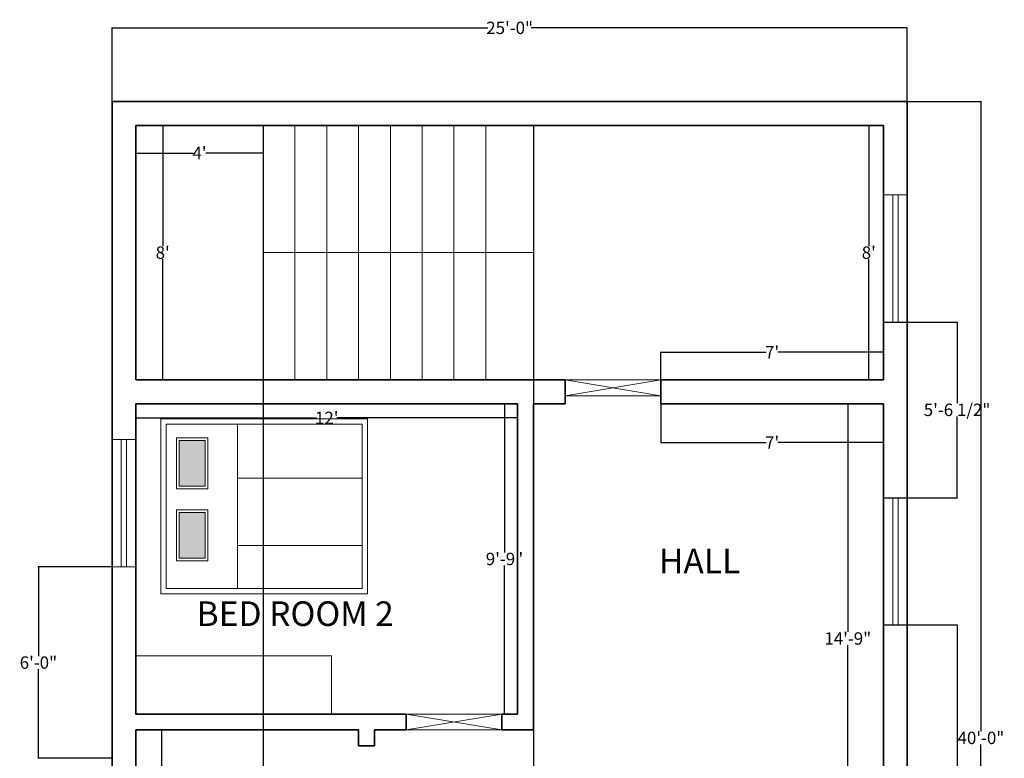
# Model space of a CAD drawing. Units: inches. Extents: x 292 to 2219, y -44 to 516.
# Tile 4 of 4: x 1035 to 1407, y 237 to 516. Entities that reach past the tile are written whole.
import ezdxf

# ---------------------------------------------------------------- set-up
doc = ezdxf.new("R2010")
doc.units = ezdxf.units.IN
doc.header["$MEASUREMENT"] = 0
for name, color, linetype, lineweight in [('A-ANNO-DIMS', 2, 'Continuous', 13), ('A-AREA-IDEN', 7, 'Continuous', 18), ('A-DOOR', 34, 'Continuous', 20), ('A-FLOR-CASE', 9, 'Continuous', 18), ('A-FLOR-STRS', 7, 'Continuous', 18), ('A-FURN', 8, 'Continuous', 18), ('A-GLAZ', 34, 'Continuous', 18), ('A-WALL', 7, 'Continuous', 35)]:
    doc.layers.add(name, color=color, linetype=linetype, lineweight=lineweight)
doc.styles.get("Standard").update_dxf_attribs({"font": 'arial.ttf'})
doc.dimstyles.get("Standard").update_dxf_attribs({"dimtxt": 4.68, "dimasz": 0.18, "dimexe": 0.18, "dimexo": 0.0625, "dimgap": 0.09, "dimtad": 0, "dimtih": 1, "dimtoh": 1, "dimdec": 0, "dimzin": 0, "dimdsep": 46, "dimlunit": 3, "dimtxsty": 'Standard', "dimcen": 0.09, "dimadec": 0, "dimazin": 0, "dimtfac": 1, "dimtdec": 0, "dimtofl": 0, "dimtmove": 0, "dimatfit": 3, "dimfxl": 1, "dimtolj": 1, "dimtzin": 0, "dimarcsym": 0})

# ---------------------------------------------------------------- blocks, each defined once
blk = doc.blocks.new('*D17')
at = {"layer": 'A-ANNO-DIMS', "color": 0, "lineweight": -2, "transparency": 16777216}
for p, q in [((1079.18, 475.82), (1089.41, 475.82)), ((1089.23, 475.64), (1089.23, 430.3)), ((1089.23, 380), (1089.23, 425.34)), ((1079.18, 379.82), (1089.41, 379.82))]:
    blk.add_line(p, q, dxfattribs=at)
at = {"layer": 'A-ANNO-DIMS', "color": 0, "transparency": 16777216}
for points in [[(1089.2, 475.64), (1089.26, 475.64), (1089.23, 475.82)], [(1089.2, 380), (1089.26, 380), (1089.23, 379.82)]]:
    blk.add_solid(points, dxfattribs=at)
at = {"layer": 'Defpoints', "color": 0, "transparency": 16777216}
for p in [(1079.11, 475.82), (1089.23, 475.82), (1079.11, 379.82)]:
    blk.add_point(p, dxfattribs=at)
at = {"layer": 'A-ANNO-DIMS', "color": 0, "transparency": 16777216, "insert": (1089.23, 427.82), "char_height": 4.68, "attachment_point": 5}
blk.add_mtext("\\A1;8'", dxfattribs=at)
blk = doc.blocks.new('*D18')
at = {"layer": 'A-ANNO-DIMS', "color": 0, "lineweight": -2, "transparency": 16777216}
for p, q in [((1079.11, 475.75), (1079.11, 465.21)), ((1127.11, 475.75), (1127.11, 465.21)), ((1079.29, 465.39), (1100.78, 465.39)), ((1126.93, 465.39), (1105.45, 465.39))]:
    blk.add_line(p, q, dxfattribs=at)
at = {"layer": 'A-ANNO-DIMS', "color": 0, "transparency": 16777216}
for points in [[(1079.29, 465.42), (1079.29, 465.36), (1079.11, 465.39)], [(1126.93, 465.42), (1126.93, 465.36), (1127.11, 465.39)]]:
    blk.add_solid(points, dxfattribs=at)
at = {"layer": 'Defpoints', "color": 0, "transparency": 16777216}
for p in [(1079.11, 475.82), (1127.11, 475.82), (1127.11, 465.39)]:
    blk.add_point(p, dxfattribs=at)
at = {"layer": 'A-ANNO-DIMS', "color": 0, "transparency": 16777216, "insert": (1103.11, 465.39), "char_height": 4.68, "attachment_point": 5}
blk.add_mtext("\\A1;4'", dxfattribs=at)
blk = doc.blocks.new('*D19')
at = {"layer": 'A-ANNO-DIMS', "color": 0, "lineweight": -2, "transparency": 16777216}
for p, q in [((1223.05, 370.82), (1217.99, 370.82)), ((1218.17, 370.64), (1218.17, 314.8)), ((1218.17, 254), (1218.17, 309.84)), ((1223.05, 253.82), (1217.99, 253.82))]:
    blk.add_line(p, q, dxfattribs=at)
at = {"layer": 'A-ANNO-DIMS', "color": 0, "transparency": 16777216}
for points in [[(1218.14, 370.64), (1218.2, 370.64), (1218.17, 370.82)], [(1218.14, 254), (1218.2, 254), (1218.17, 253.82)]]:
    blk.add_solid(points, dxfattribs=at)
at = {"layer": 'Defpoints', "color": 0, "transparency": 16777216}
for p in [(1218.17, 370.82), (1223.11, 370.82), (1223.11, 253.82)]:
    blk.add_point(p, dxfattribs=at)
at = {"layer": 'A-ANNO-DIMS', "color": 0, "transparency": 16777216, "insert": (1218.17, 312.32), "char_height": 4.68, "attachment_point": 5}
blk.add_mtext('\\A1;9\'-9"', dxfattribs=at)
blk = doc.blocks.new('*D20')
at = {"layer": 'A-ANNO-DIMS', "color": 0, "lineweight": -2, "transparency": 16777216}
for p, q in [((1079.11, 370.75), (1079.11, 365.33)), ((1223.11, 370.75), (1223.11, 365.33)), ((1079.29, 365.51), (1147.27, 365.51)), ((1222.93, 365.51), (1154.95, 365.51))]:
    blk.add_line(p, q, dxfattribs=at)
at = {"layer": 'A-ANNO-DIMS', "color": 0, "transparency": 16777216}
for points in [[(1079.29, 365.54), (1079.29, 365.48), (1079.11, 365.51)], [(1222.93, 365.54), (1222.93, 365.48), (1223.11, 365.51)]]:
    blk.add_solid(points, dxfattribs=at)
at = {"layer": 'Defpoints', "color": 0, "transparency": 16777216}
for p in [(1079.11, 370.82), (1223.11, 370.82), (1223.11, 365.51)]:
    blk.add_point(p, dxfattribs=at)
at = {"layer": 'A-ANNO-DIMS', "color": 0, "transparency": 16777216, "insert": (1151.11, 365.51), "char_height": 4.68, "attachment_point": 5}
blk.add_mtext("\\A1;12'", dxfattribs=at)
blk = doc.blocks.new('*D21')
at = {"layer": 'A-ANNO-DIMS', "color": 0, "lineweight": -2, "transparency": 16777216}
for p, q in [((1079.18, 247.82), (1088.93, 247.82)), ((1088.75, 247.64), (1088.75, 223.3)), ((1088.75, 194), (1088.75, 218.34)), ((1079.18, 193.82), (1088.93, 193.82))]:
    blk.add_line(p, q, dxfattribs=at)
at = {"layer": 'A-ANNO-DIMS', "color": 0, "transparency": 16777216}
for points in [[(1088.72, 247.64), (1088.78, 247.64), (1088.75, 247.82)], [(1088.72, 194), (1088.78, 194), (1088.75, 193.82)]]:
    blk.add_solid(points, dxfattribs=at)
at = {"layer": 'Defpoints', "color": 0, "transparency": 16777216}
for p in [(1079.11, 247.82), (1088.75, 247.82), (1079.11, 193.82)]:
    blk.add_point(p, dxfattribs=at)
at = {"layer": 'A-ANNO-DIMS', "color": 0, "transparency": 16777216, "insert": (1088.75, 220.82), "char_height": 4.68, "attachment_point": 5}
blk.add_mtext('\\A1;4\'-6"', dxfattribs=at)
blk = doc.blocks.new('*D33')
at = {"layer": 'A-ANNO-DIMS', "color": 0, "lineweight": -2, "transparency": 16777216}
for p, q in [((1277.11, 370.75), (1277.11, 356.01)), ((1361.11, 370.75), (1361.11, 356.01)), ((1277.29, 356.19), (1316.89, 356.19)), ((1360.93, 356.19), (1321.34, 356.19))]:
    blk.add_line(p, q, dxfattribs=at)
at = {"layer": 'A-ANNO-DIMS', "color": 0, "transparency": 16777216}
for points in [[(1277.29, 356.22), (1277.29, 356.16), (1277.11, 356.19)], [(1360.93, 356.22), (1360.93, 356.16), (1361.11, 356.19)]]:
    blk.add_solid(points, dxfattribs=at)
at = {"layer": 'Defpoints', "color": 0, "transparency": 16777216}
for p in [(1277.11, 370.82), (1361.11, 370.82), (1361.11, 356.19)]:
    blk.add_point(p, dxfattribs=at)
at = {"layer": 'A-ANNO-DIMS', "color": 0, "transparency": 16777216, "insert": (1319.11, 356.19), "char_height": 4.68, "attachment_point": 5}
blk.add_mtext("\\A1;7'", dxfattribs=at)
blk = doc.blocks.new('*D34')
at = {"layer": 'A-ANNO-DIMS', "color": 0, "lineweight": -2, "transparency": 16777216}
for p, q in [((1361.05, 370.82), (1347.49, 370.82)), ((1347.67, 370.64), (1347.67, 284.8)), ((1347.67, 194), (1347.67, 279.84)), ((1361.05, 193.82), (1347.49, 193.82))]:
    blk.add_line(p, q, dxfattribs=at)
at = {"layer": 'A-ANNO-DIMS', "color": 0, "transparency": 16777216}
for points in [[(1347.64, 370.64), (1347.7, 370.64), (1347.67, 370.82)], [(1347.64, 194), (1347.7, 194), (1347.67, 193.82)]]:
    blk.add_solid(points, dxfattribs=at)
at = {"layer": 'Defpoints', "color": 0, "transparency": 16777216}
for p in [(1347.67, 370.82), (1361.11, 370.82), (1361.11, 193.82)]:
    blk.add_point(p, dxfattribs=at)
at = {"layer": 'A-ANNO-DIMS', "color": 0, "transparency": 16777216, "insert": (1347.67, 282.32), "char_height": 4.68, "attachment_point": 5}
blk.add_mtext('\\A1;14\'-9"', dxfattribs=at)
blk = doc.blocks.new('*D35')
at = {"layer": 'A-ANNO-DIMS', "color": 0, "lineweight": -2, "transparency": 16777216}
for p, q in [((1277.11, 379.88), (1277.11, 390.47)), ((1277.29, 390.29), (1316.89, 390.29)), ((1360.93, 390.29), (1321.34, 390.29)), ((1361.11, 379.88), (1361.11, 390.47))]:
    blk.add_line(p, q, dxfattribs=at)
at = {"layer": 'A-ANNO-DIMS', "color": 0, "transparency": 16777216}
for points in [[(1277.29, 390.32), (1277.29, 390.26), (1277.11, 390.29)], [(1360.93, 390.32), (1360.93, 390.26), (1361.11, 390.29)]]:
    blk.add_solid(points, dxfattribs=at)
at = {"layer": 'Defpoints', "color": 0, "transparency": 16777216}
for p in [(1361.11, 390.29), (1277.11, 379.82), (1361.11, 379.82)]:
    blk.add_point(p, dxfattribs=at)
at = {"layer": 'A-ANNO-DIMS', "color": 0, "transparency": 16777216, "insert": (1319.11, 390.29), "char_height": 4.68, "attachment_point": 5}
blk.add_mtext("\\A1;7'", dxfattribs=at)
blk = doc.blocks.new('*D36')
at = {"layer": 'A-ANNO-DIMS', "color": 0, "lineweight": -2, "transparency": 16777216}
for p, q in [((1361.05, 475.82), (1355.4, 475.82)), ((1355.58, 475.64), (1355.58, 430.3)), ((1355.58, 380), (1355.58, 425.34)), ((1361.05, 379.82), (1355.4, 379.82))]:
    blk.add_line(p, q, dxfattribs=at)
at = {"layer": 'A-ANNO-DIMS', "color": 0, "transparency": 16777216}
for points in [[(1355.55, 475.64), (1355.61, 475.64), (1355.58, 475.82)], [(1355.55, 380), (1355.61, 380), (1355.58, 379.82)]]:
    blk.add_solid(points, dxfattribs=at)
at = {"layer": 'Defpoints', "color": 0, "transparency": 16777216}
for p in [(1355.58, 475.82), (1361.11, 475.82), (1361.11, 379.82)]:
    blk.add_point(p, dxfattribs=at)
at = {"layer": 'A-ANNO-DIMS', "color": 0, "transparency": 16777216, "insert": (1355.58, 427.82), "char_height": 4.68, "attachment_point": 5}
blk.add_mtext("\\A1;8'", dxfattribs=at)
blk = doc.blocks.new('BED-DOUBLE')
h = blk.add_hatch(color=256)
h.dxf.hatch_style = 1
h.paths.add_polyline_path([(6.9, 40.51), (16.75, 40.51), (16.75, 57.79), (6.9, 57.79)])
h.paths.add_polyline_path([(16.75, 30.67), (6.9, 30.67), (6.9, 13.4), (16.75, 13.4)])
for p, q in [((0, 0), (0, 66)), ((0, 66), (78, 66)), ((2, 64), (76, 64)), ((2, 2), (2, 64)), ((29, 2), (29, 64)), ((76, 64), (76, 2)), ((78, 66), (78, 0)), ((76, 43.53), (29, 43.53)), ((76, 18.22), (29, 18.22)), ((78, 0), (0, 0)), ((76, 2), (2, 2))]:
    blk.add_line(p, q)
for points in [[(5.9, 58.79), (17.75, 58.79), (17.75, 39.51), (5.9, 39.51)], [(6.9, 57.79), (16.75, 57.79), (16.75, 40.51), (6.9, 40.51)], [(5.9, 31.67), (17.75, 31.67), (17.75, 12.4), (5.9, 12.4)], [(6.9, 30.67), (16.75, 30.67), (16.75, 13.4), (6.9, 13.4)]]:
    blk.add_lwpolyline(points, close=True)
blk = doc.blocks.new('WIN-48')
for p, q in [((0, 48), (9, 48)), ((0, 0), (0, 48)), ((3.5, 48), (3.5, 0)), ((5.5, 48), (5.5, 0)), ((9, 48), (9, 0)), ((9, 0), (0, 0))]:
    blk.add_line(p, q)
blk = doc.blocks.new('DOOR-36')
for p, q in [((0, 36), (6, 36)), ((0, 0), (6, 36)), ((6, 0), (0, 36)), ((0, 36), (0, 0)), ((6, 36), (6, 0)), ((0, 0), (6, 0))]:
    blk.add_line(p, q)
blk = doc.blocks.new('BEDROOM-CABINET')
blk.add_lwpolyline([(0, 21.98), (73.86, 21.98), (73.86, 0), (0, 0)], close=True)
blk = doc.blocks.new('*D69')
at = {"layer": 'A-ANNO-DIMS', "color": 0, "lineweight": -2, "transparency": 16777216}
for p, q in [((1070.05, 309.31), (1042.16, 309.31)), ((1042.34, 309.13), (1042.34, 275.7)), ((1042.34, 237.32), (1042.34, 270.75)), ((1070.05, 237.14), (1042.16, 237.14))]:
    blk.add_line(p, q, dxfattribs=at)
at = {"layer": 'A-ANNO-DIMS', "color": 0, "transparency": 16777216}
for points in [[(1042.31, 309.13), (1042.37, 309.13), (1042.34, 309.31)], [(1042.31, 237.32), (1042.37, 237.32), (1042.34, 237.14)]]:
    blk.add_solid(points, dxfattribs=at)
at = {"layer": 'Defpoints', "color": 0, "transparency": 16777216}
for p in [(1042.34, 309.31), (1070.11, 309.31), (1070.11, 237.14)]:
    blk.add_point(p, dxfattribs=at)
at = {"layer": 'A-ANNO-DIMS', "color": 0, "transparency": 16777216, "insert": (1042.34, 273.23), "char_height": 4.68, "attachment_point": 5}
blk.add_mtext('\\A1;6\'-0"', dxfattribs=at)
blk = doc.blocks.new('*D71')
at = {"layer": 'A-ANNO-DIMS', "color": 0, "lineweight": -2, "transparency": 16777216}
for p, q in [((1361.18, 287.41), (1389.07, 287.41)), ((1388.89, 287.23), (1388.89, 220.75)), ((1388.89, 149.26), (1388.89, 215.73)), ((1361.18, 149.08), (1389.07, 149.08))]:
    blk.add_line(p, q, dxfattribs=at)
at = {"layer": 'A-ANNO-DIMS', "color": 0, "transparency": 16777216}
for points in [[(1388.86, 287.23), (1388.92, 287.23), (1388.89, 287.41)], [(1388.86, 149.26), (1388.92, 149.26), (1388.89, 149.08)]]:
    blk.add_solid(points, dxfattribs=at)
at = {"layer": 'Defpoints', "color": 0, "transparency": 16777216}
for p in [(1361.11, 287.41), (1361.11, 149.08), (1388.89, 149.08)]:
    blk.add_point(p, dxfattribs=at)
at = {"layer": 'A-ANNO-DIMS', "color": 0, "transparency": 16777216, "insert": (1388.89, 218.24), "char_height": 4.68, "attachment_point": 5}
blk.add_mtext('\\A1;11\'-6 1/2"', dxfattribs=at)
blk = doc.blocks.new('*D72')
at = {"layer": 'A-ANNO-DIMS', "color": 0, "lineweight": -2, "transparency": 16777216}
for p, q in [((1361.18, 401.66), (1389.07, 401.66)), ((1388.89, 401.48), (1388.89, 371.05)), ((1388.89, 335.59), (1388.89, 366.03)), ((1361.18, 335.41), (1389.07, 335.41))]:
    blk.add_line(p, q, dxfattribs=at)
at = {"layer": 'A-ANNO-DIMS', "color": 0, "transparency": 16777216}
for points in [[(1388.86, 401.48), (1388.92, 401.48), (1388.89, 401.66)], [(1388.86, 335.59), (1388.92, 335.59), (1388.89, 335.41)]]:
    blk.add_solid(points, dxfattribs=at)
at = {"layer": 'Defpoints', "color": 0, "transparency": 16777216}
for p in [(1361.11, 401.66), (1361.11, 335.41), (1388.89, 335.41)]:
    blk.add_point(p, dxfattribs=at)
at = {"layer": 'A-ANNO-DIMS', "color": 0, "transparency": 16777216, "insert": (1388.89, 368.54), "char_height": 4.68, "attachment_point": 5}
blk.add_mtext('\\A1;5\'-6 1/2"', dxfattribs=at)
blk = doc.blocks.new('*D73')
at = {"layer": 'A-ANNO-DIMS', "color": 0, "lineweight": -2, "transparency": 16777216}
for p, q in [((1127.11, 475.75), (1127.11, -23.14)), ((1229.11, 475.75), (1229.11, -23.14)), ((1127.29, -22.96), (1171.8, -22.96)), ((1228.93, -22.96), (1184.43, -22.96))]:
    blk.add_line(p, q, dxfattribs=at)
at = {"layer": 'A-ANNO-DIMS', "color": 0, "transparency": 16777216}
for points in [[(1127.29, -22.93), (1127.29, -22.99), (1127.11, -22.96)], [(1228.93, -22.93), (1228.93, -22.99), (1229.11, -22.96)]]:
    blk.add_solid(points, dxfattribs=at)
at = {"layer": 'Defpoints', "color": 0, "transparency": 16777216}
for p in [(1127.11, 475.82), (1229.11, 475.82), (1229.11, -22.96)]:
    blk.add_point(p, dxfattribs=at)
at = {"layer": 'A-ANNO-DIMS', "color": 0, "transparency": 16777216, "insert": (1178.11, -22.96), "char_height": 4.68, "attachment_point": 5}
blk.add_mtext('\\A1;8\'-6"', dxfattribs=at)
blk = doc.blocks.new('*D74')
at = {"layer": 'A-ANNO-DIMS', "color": 0, "lineweight": -2, "transparency": 16777216}
for p, q in [((1070.11, 484.88), (1070.11, 512.77)), ((1070.29, 512.59), (1211.94, 512.59)), ((1369.93, 512.59), (1228.28, 512.59)), ((1370.11, 484.88), (1370.11, 512.77))]:
    blk.add_line(p, q, dxfattribs=at)
at = {"layer": 'A-ANNO-DIMS', "color": 0, "transparency": 16777216}
for points in [[(1070.29, 512.62), (1070.29, 512.56), (1070.11, 512.59)], [(1369.93, 512.62), (1369.93, 512.56), (1370.11, 512.59)]]:
    blk.add_solid(points, dxfattribs=at)
at = {"layer": 'Defpoints', "color": 0, "transparency": 16777216}
for p in [(1370.11, 512.59), (1070.11, 484.82), (1370.11, 484.82)]:
    blk.add_point(p, dxfattribs=at)
at = {"layer": 'A-ANNO-DIMS', "color": 0, "transparency": 16777216, "insert": (1220.11, 512.59), "char_height": 4.68, "attachment_point": 5}
blk.add_mtext('\\A1;25\'-0"', dxfattribs=at)
blk = doc.blocks.new('*D75')
at = {"layer": 'A-ANNO-DIMS', "color": 0, "lineweight": -2, "transparency": 16777216}
for p, q in [((1370.18, 484.82), (1398.07, 484.82)), ((1397.89, 484.64), (1397.89, 247.3)), ((1397.89, 5), (1397.89, 242.34)), ((1370.18, 4.82), (1398.07, 4.82))]:
    blk.add_line(p, q, dxfattribs=at)
at = {"layer": 'A-ANNO-DIMS', "color": 0, "transparency": 16777216}
for points in [[(1397.86, 484.64), (1397.92, 484.64), (1397.89, 484.82)], [(1397.86, 5), (1397.92, 5), (1397.89, 4.82)]]:
    blk.add_solid(points, dxfattribs=at)
at = {"layer": 'Defpoints', "color": 0, "transparency": 16777216}
for p in [(1370.11, 484.82), (1397.89, 484.82), (1370.11, 4.82)]:
    blk.add_point(p, dxfattribs=at)
at = {"layer": 'A-ANNO-DIMS', "color": 0, "transparency": 16777216, "insert": (1397.89, 244.82), "char_height": 4.68, "attachment_point": 5}
blk.add_mtext('\\A1;40\'-0"', dxfattribs=at)

msp = doc.modelspace()

# ---------------------------------------------------------------- linework, layer by layer
at = {"layer": 'A-FLOR-STRS'}
for p, q in [((1127.11, 379.82), (1127.11, 475.82)), ((1139.11, 379.82), (1139.11, 475.82)), ((1151.11, 379.82), (1151.11, 475.82)), ((1163.11, 379.82), (1163.11, 475.82)), ((1175.11, 379.82), (1175.11, 475.82)), ((1187.11, 379.82), (1187.11, 475.82)), ((1199.11, 379.82), (1199.11, 475.82)), ((1211.11, 379.82), (1211.11, 475.82)), ((1229.11, 379.82), (1229.11, 475.82)), ((1127.11, 427.82), (1229.11, 427.82))]:
    msp.add_line(p, q, dxfattribs=at)
at = {"layer": 'A-WALL'}
for p, q in [((1070.11, 4.82), (1070.11, 484.82)), ((1070.11, 484.82), (1370.11, 484.82)), ((1370.11, 484.82), (1370.11, 4.82)), ((1079.11, 475.82), (1361.11, 475.82)), ((1079.11, 379.82), (1079.11, 475.82)), ((1079.11, 379.82), (1079.11, 475.82)), ((1361.11, 475.82), (1361.11, 379.82)), ((1079.11, 379.82), (1241.11, 379.82)), ((1241.11, 370.82), (1241.11, 379.82)), ((1277.11, 370.82), (1277.11, 379.82)), ((1277.11, 379.82), (1361.11, 379.82)), ((1079.11, 253.82), (1079.11, 370.82)), ((1079.11, 253.82), (1079.11, 370.82)), ((1079.11, 370.82), (1223.11, 370.82)), ((1223.11, 253.82), (1223.11, 370.82)), ((1229.11, 247.82), (1229.11, 370.82)), ((1229.11, 370.82), (1241.11, 370.82)), ((1277.11, 370.82), (1361.11, 370.82)), ((1361.11, 370.82), (1361.11, 193.82)), ((1079.11, 253.82), (1181.11, 253.82)), ((1181.11, 253.82), (1181.11, 247.82)), ((1217.11, 253.82), (1217.11, 247.82)), ((1217.11, 253.82), (1223.11, 253.82)), ((1079.11, 247.82), (1163.11, 247.82)), ((1079.11, 193.82), (1079.11, 247.82)), ((1079.11, 199.82), (1079.11, 247.82)), ((1163.11, 241.82), (1163.11, 247.82)), ((1169.11, 247.82), (1181.11, 247.82)), ((1169.11, 241.82), (1169.11, 247.82)), ((1217.11, 247.82), (1229.11, 247.82)), ((1163.11, 241.82), (1169.11, 241.82))]:
    msp.add_line(p, q, dxfattribs=at)

# ---------------------------------------------------------------- block references
at = {"layer": 'A-DOOR'}
for p, rotation in [((1277.11, 373.82), 90.00000000000038), ((1217.11, 247.82), 90.00000000000075)]:
    msp.add_blockref('DOOR-36', p, dxfattribs=dict(at, rotation=rotation))
at = {"layer": 'A-FLOR-CASE'}
msp.add_blockref('BEDROOM-CABINET', (1079.11, 253.82), dxfattribs=at)
at = {"layer": 'A-FURN'}
msp.add_blockref('BED-DOUBLE', (1088.51, 299.2), dxfattribs=at)
at = {"layer": 'A-GLAZ'}
for p in [(1361.11, 401.66), (1070.11, 309.31), (1361.11, 287.41)]:
    msp.add_blockref('WIN-48', p, dxfattribs=at)

# ---------------------------------------------------------------- texts
at = {"layer": 'A-AREA-IDEN'}
for s, p in [('HALL', (1276.43, 306.85)), ('BED ROOM 2', (1102.03, 287.03))]:
    msp.add_text(s, height=9.289, dxfattribs=at).set_placement(p)

# ---------------------------------------------------------------- dimensions: what is measured, and where the dimension line sits
at = {"layer": 'A-ANNO-DIMS'}
for base, p1, p2, override, picture, middle in [((1370.11, 512.59), (1070.11, 484.82), (1370.11, 484.82), {"dimdec": 1, "dimlfac": 1, "dimrnd": 0, "dimzin": 1, "dimdsep": 46, "dimlunit": 4, "dimfrac": 2}, '*D74', (1220.11, 512.59)), ((1127.11, 465.39), (1079.11, 475.82), (1127.11, 475.82), {"dimclrd": 0, "dimclre": 0, "dimclrt": 0}, '*D18', (1103.11, 465.39)), ((1229.11, -22.96), (1127.11, 475.82), (1229.11, 475.82), {"dimdec": 1, "dimlfac": 1, "dimrnd": 0, "dimzin": 1, "dimdsep": 46, "dimlunit": 4, "dimfrac": 2}, '*D73', (1178.11, -22.96)), ((1361.11, 390.29), (1277.11, 379.82), (1361.11, 379.82), {"dimclrd": 0, "dimclre": 0, "dimclrt": 0}, '*D35', (1319.11, 390.29)), ((1223.11, 365.51), (1079.11, 370.82), (1223.11, 370.82), {"dimclrd": 0, "dimclre": 0, "dimclrt": 0}, '*D20', (1151.11, 365.51)), ((1361.11, 356.19), (1277.11, 370.82), (1361.11, 370.82), {"dimclrd": 0, "dimclre": 0, "dimclrt": 0}, '*D33', (1319.11, 356.19))]:
    dim = msp.add_linear_dim(base=base, p1=p1, p2=p2, dimstyle='Standard', override=override, dxfattribs=at)
    dim.commit()
    dim.dimension.update_dxf_attribs({"geometry": picture, "text_midpoint": middle})
for base, p1, p2, angle, override, picture, middle in [((1397.89, 484.82), (1370.11, 4.82), (1370.11, 484.82), 90, {"dimdec": 1, "dimlfac": 1, "dimrnd": 0, "dimzin": 1, "dimdsep": 46, "dimlunit": 4, "dimfrac": 2}, '*D75', (1397.89, 244.82)), ((1089.23, 475.82), (1079.11, 379.82), (1079.11, 475.82), 90, {"dimclrd": 0, "dimclre": 0, "dimclrt": 0}, '*D17', (1089.23, 427.82)), ((1355.58, 475.82), (1361.11, 379.82), (1361.11, 475.82), 90, {"dimclrd": 0, "dimclre": 0, "dimclrt": 0}, '*D36', (1355.58, 427.82)), ((1388.8879, 335.4115), (1361.1129, 401.6618), (1361.1129, 335.4115), 270, {"dimdec": 1, "dimlfac": 1, "dimrnd": 0, "dimzin": 1, "dimdsep": 46, "dimlunit": 4, "dimfrac": 2}, '*D72', (1388.8879, 368.5366)), ((1218.17, 370.82), (1223.11, 253.82), (1223.11, 370.82), 90, {"dimclrd": 0, "dimclre": 0, "dimclrt": 0}, '*D19', (1218.17, 312.32)), ((1347.67, 370.82), (1361.11, 193.82), (1361.11, 370.82), 90, {"dimclrd": 0, "dimclre": 0, "dimclrt": 0}, '*D34', (1347.67, 282.32)), ((1042.34, 309.31), (1070.11, 237.14), (1070.11, 309.31), 90, {"dimdec": 1, "dimlfac": 1, "dimrnd": 0, "dimzin": 1, "dimdsep": 46, "dimlunit": 4, "dimfrac": 2}, '*D69', (1042.34, 273.23)), ((1388.89, 149.08), (1361.11, 287.41), (1361.11, 149.08), 270, {"dimdec": 1, "dimlfac": 1, "dimrnd": 0, "dimzin": 1, "dimdsep": 46, "dimlunit": 4, "dimfrac": 2}, '*D71', (1388.89, 218.24)), ((1088.75, 247.82), (1079.11, 193.82), (1079.11, 247.82), 90, {"dimclrd": 0, "dimclre": 0, "dimclrt": 0}, '*D21', (1088.75, 220.82))]:
    dim = msp.add_linear_dim(base=base, p1=p1, p2=p2, angle=angle, dimstyle='Standard', override=override, dxfattribs=at)
    dim.commit()
    dim.dimension.update_dxf_attribs({"geometry": picture, "text_midpoint": middle})

doc.saveas('drawing.dxf')
